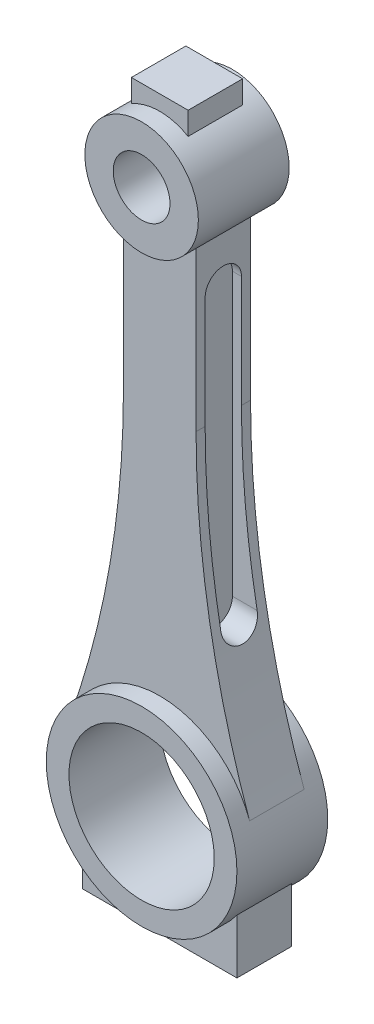
from build123d import *

# Parameters (mm, degrees)
ROD_PROFILE_SKETCH_R   = 12.5
ROD_PROFILE_SKETCH_R_2 = 6.25
ROD_BODY_DEPTH         = 10
ROD_PROFILE_SKETCH_R_3 = 21
ROD_PROFILE_SKETCH_R_4 = 16
ROD_BODY_2_DEPTH       = 10
EYE_BOSS_DEPTH         = 6
WEB_START              = 6
WEB_RECESS_CUT_DEPTH   = 132.802456026


with BuildPart() as part:
    # Rod Profile Sketch → Rod Body (new, symmetric)
    with BuildSketch(Plane.XY):
        with Locations((0, 120)):
            Circle(ROD_PROFILE_SKETCH_R)
        with Locations((0, 120)):
            Circle(ROD_PROFILE_SKETCH_R_2, mode=Mode.SUBTRACT)
    extrude(amount=ROD_BODY_DEPTH, both=True)



with BuildPart() as body_2:
    # Rod Profile Sketch → Rod Body 2 (new, symmetric)
    with BuildSketch(Plane.XY):
        Circle(ROD_PROFILE_SKETCH_R_3)
        Circle(ROD_PROFILE_SKETCH_R_4, mode=Mode.SUBTRACT)
    extrude(amount=ROD_BODY_2_DEPTH, both=True)


with BuildPart() as part_1:
    add(part.part)

    add(body_2.part)  # Eye Boss merges body 2
    # Sketch1_3 → Eye Boss (add, symmetric)
    with BuildSketch(Plane.XY):
        with BuildLine():
            Line((-8, 110.395313644), (-8, 75.395313644))
            ThreePointArc((-8, 75.395313644), (-10.96842855, 40.709642053), (-19.787382488, 7.032744434))
            ThreePointArc((-19.787382488, 7.032744434), (0, 21), (19.787382488, 7.032744434))
            ThreePointArc((19.787382488, 7.032744434), (10.96842855, 40.709642053), (8, 75.395313644))
            Line((8, 75.395313644), (8, 110.395313644))
            ThreePointArc((8, 110.395313644), (0, 107.5), (-8, 110.395313644))
        make_face()
        with BuildLine():
            Line((-6.25, 135.825317547), (-6.25, 130.825317547))
            ThreePointArc((-6.25, 130.825317547), (0, 132.5), (6.25, 130.825317547))
            Line((6.25, 130.825317547), (6.25, 135.825317547))
            Line((6.25, 135.825317547), (-6.25, 135.825317547))
        make_face()
        with BuildLine():
            ThreePointArc((17, -12.328828006), (0, -21), (-17, -12.328828006))
            Line((-17, -12.328828006), (-17, -24.328828006))
            Line((-17, -24.328828006), (17, -24.328828006))
            Line((17, -24.328828006), (17, -12.328828006))
        make_face()
    extrude(amount=EYE_BOSS_DEPTH, both=True)

    # Web Recess Sketch → Web Recess Cut (cut, through all)
    with BuildSketch(Plane(origin=(0, 0, 0), x_dir=(0, 0, -1), z_dir=(1, 0, 0)).offset(WEB_START)):
        with BuildLine():
            Line((4, 100), (4, 38))
            ThreePointArc((4, 38), (0, 34), (-4, 38))
            Line((-4, 38), (-4, 100))
            ThreePointArc((-4, 100), (0, 104), (4, 100))
        make_face()
    web_recess_cut = extrude(amount=WEB_RECESS_CUT_DEPTH, mode=Mode.SUBTRACT)

    # Web Recess Mirror: Web Recess Cut across plane
    add(web_recess_cut.mirror(Plane(origin=(0, 0, 0), x_dir=(0, 0, 1), z_dir=(1, 0, 0))), mode=Mode.SUBTRACT)


solid = part_1.part
